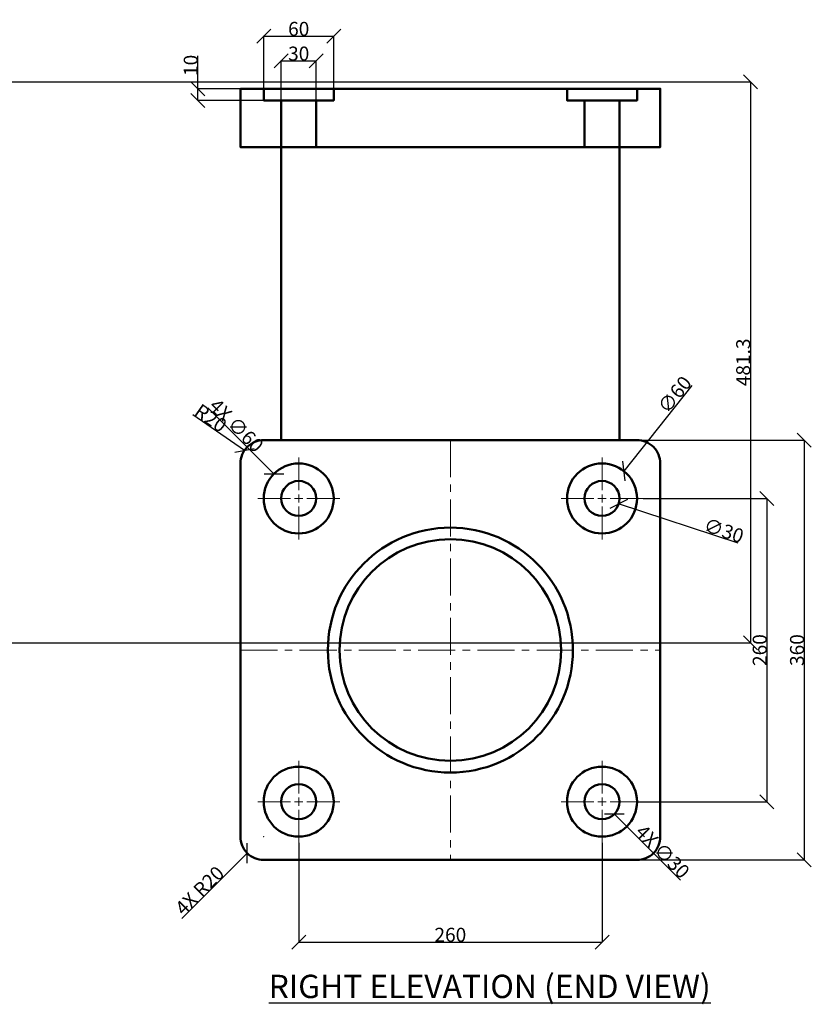
# Model space of a CAD drawing. Units: millimetres. Extents: x 509 to 2033, y 349 to 1731.
# Tile 2 of 2: x 1355 to 2033, y 349 to 1193. Entities that reach past the tile are written whole.
import ezdxf

# ---------------------------------------------------------------- set-up
doc = ezdxf.new("R2010")
doc.units = ezdxf.units.MM
doc.header["$MEASUREMENT"] = 0
doc.linetypes.add('CENTER', pattern=[50.8, 31.75, -6.35, 6.35, -6.35])
for name, color, linetype, lineweight in [('M-CNTR', 1, 'CENTER', 18), ('M-DIMS', 2, 'Continuous', 25), ('M-OUTL', 7, 'Continuous', 50), ('M-TEXT', 7, 'Continuous', 25)]:
    doc.layers.add(name, color=color, linetype=linetype, lineweight=lineweight)
doc.styles.get("Standard").update_dxf_attribs({"font": 'arial.ttf'})
doc.dimstyles.get("Standard").update_dxf_attribs({"dimtxt": 12, "dimasz": 12, "dimexe": 0.18, "dimexo": 0.0625, "dimgap": 0.09, "dimtad": 1, "dimdec": 0, "dimzin": 0, "dimdsep": 46, "dimtxsty": 'Standard', "dimblk": 'OBLIQUE', "dimcen": 0.09, "dimclre": 251, "dimadec": 0, "dimazin": 0, "dimtfac": 1, "dimtdec": 0, "dimtofl": 0, "dimtmove": 0, "dimatfit": 3, "dimfxl": 1, "dimtolj": 1, "dimtzin": 0, "dimarcsym": 0})

# ---------------------------------------------------------------- blocks, each defined once
blk = doc.blocks.new('*U6')
at = {"layer": 'M-CNTR', "color": 0, "transparency": 16777216}
for p, q in [((0, 7), (0, 35.12)), ((-35.12, 0), (-7, 0)), ((7, 0), (35.12, 0)), ((0, -35.12), (0, -7))]:
    blk.add_line(p, q, dxfattribs=at)
at = {"layer": 'M-CNTR', "color": 0, "linetype": 'Continuous', "transparency": 16777216}
for p, q in [((-3.5, 0), (3.5, 0)), ((0, -3.5), (0, 3.5))]:
    blk.add_line(p, q, dxfattribs=at)
blk = doc.blocks.new('*U7')
at = {"layer": 'M-CNTR', "color": 0, "transparency": 16777216}
for p, q in [((0, 7), (0, 35.12)), ((-35.12, 0), (-7, 0)), ((7, 0), (35.12, 0)), ((0, -35.12), (0, -7))]:
    blk.add_line(p, q, dxfattribs=at)
at = {"layer": 'M-CNTR', "color": 0, "linetype": 'Continuous', "transparency": 16777216}
for p, q in [((-3.5, 0), (3.5, 0)), ((0, -3.5), (0, 3.5))]:
    blk.add_line(p, q, dxfattribs=at)
blk = doc.blocks.new('*U8')
at = {"layer": 'M-CNTR', "color": 0, "transparency": 16777216}
for p, q in [((0, 7), (0, 35.12)), ((-35.12, 0), (-7, 0)), ((7, 0), (35.12, 0)), ((0, -35.12), (0, -7))]:
    blk.add_line(p, q, dxfattribs=at)
at = {"layer": 'M-CNTR', "color": 0, "linetype": 'Continuous', "transparency": 16777216}
for p, q in [((-3.5, 0), (3.5, 0)), ((0, -3.5), (0, 3.5))]:
    blk.add_line(p, q, dxfattribs=at)
blk = doc.blocks.new('*U9')
at = {"layer": 'M-CNTR', "color": 0, "transparency": 16777216}
for p, q in [((0, 7), (0, 35.12)), ((-35.12, 0), (-7, 0)), ((7, 0), (35.12, 0)), ((0, -35.12), (0, -7))]:
    blk.add_line(p, q, dxfattribs=at)
at = {"layer": 'M-CNTR', "color": 0, "linetype": 'Continuous', "transparency": 16777216}
for p, q in [((-3.5, 0), (3.5, 0)), ((0, -3.5), (0, 3.5))]:
    blk.add_line(p, q, dxfattribs=at)
blk = doc.blocks.new('_Oblique')
at = {"color": 0, "linetype": 'ByBlock', "lineweight": -2}
blk.add_line((-0.5, -0.5), (0.5, 0.5), dxfattribs=at)
blk = doc.blocks.new('*D25')
at = {"layer": 'Defpoints', "color": 0, "transparency": 16777216}
for p in [(1507.36, 1133.76), (1563.7, 1133.76), (1563.7, 1123.76)]:
    blk.add_point(p, dxfattribs=at)
at = {"layer": 'M-DIMS', "color": 0, "lineweight": -2, "transparency": 16777216}
for p, q in [((1507.36, 1133.76), (1507.36, 1161.96)), ((1563.64, 1133.76), (1507.18, 1133.76)), ((1507.36, 1123.76), (1507.36, 1133.76)), ((1563.64, 1123.76), (1507.18, 1123.76))]:
    blk.add_line(p, q, dxfattribs=at)
at = {"layer": 'M-DIMS', "color": 0, "lineweight": -2, "transparency": 16777216, "xscale": 12, "yscale": 12, "zscale": 12}
for p, rotation in [((1507.36, 1133.76), 90), ((1507.36, 1123.76), 270)]:
    blk.add_blockref('_Oblique', p, dxfattribs=dict(at, rotation=rotation))
at = {"layer": 'M-DIMS', "color": 0, "transparency": 16777216, "insert": (1501.14, 1153.86), "char_height": 12, "attachment_point": 5, "rotation": 90}
blk.add_mtext('\\A1;10', dxfattribs=at)
blk = doc.blocks.new('*D26')
at = {"layer": 'Defpoints', "color": 0, "transparency": 16777216}
for p in [(1623.7, 1178.95), (1563.7, 1133.76), (1623.7, 1133.76)]:
    blk.add_point(p, dxfattribs=at)
at = {"layer": 'M-DIMS', "color": 0, "lineweight": -2, "transparency": 16777216}
for p, q in [((1563.7, 1133.82), (1563.7, 1179.13)), ((1563.7, 1178.95), (1623.7, 1178.95)), ((1623.7, 1133.82), (1623.7, 1179.13))]:
    blk.add_line(p, q, dxfattribs=at)
at = {"layer": 'M-DIMS', "color": 0, "lineweight": -2, "transparency": 16777216, "xscale": 12, "yscale": 12, "zscale": 12, "rotation": 180}
blk.add_blockref('_Oblique', (1563.7, 1178.95), dxfattribs=at)
at = {"layer": 'M-DIMS', "color": 0, "lineweight": -2, "transparency": 16777216, "xscale": 12, "yscale": 12, "zscale": 12}
blk.add_blockref('_Oblique', (1623.7, 1178.95), dxfattribs=at)
at = {"layer": 'M-DIMS', "color": 0, "transparency": 16777216, "insert": (1593.7, 1185.16), "char_height": 12, "attachment_point": 5}
blk.add_mtext('\\A1;60', dxfattribs=at)
blk = doc.blocks.new('*D27')
at = {"layer": 'Defpoints', "color": 0, "transparency": 16777216}
for p in [(1608.7, 1157.75), (1578.7, 1123.76), (1608.7, 1123.76)]:
    blk.add_point(p, dxfattribs=at)
at = {"layer": 'M-DIMS', "color": 0, "lineweight": -2, "transparency": 16777216}
for p, q in [((1578.7, 1123.82), (1578.7, 1157.93)), ((1578.7, 1157.75), (1608.7, 1157.75)), ((1608.7, 1123.82), (1608.7, 1157.93))]:
    blk.add_line(p, q, dxfattribs=at)
at = {"layer": 'M-DIMS', "color": 0, "lineweight": -2, "transparency": 16777216, "xscale": 12, "yscale": 12, "zscale": 12, "rotation": 180}
blk.add_blockref('_Oblique', (1578.7, 1157.75), dxfattribs=at)
at = {"layer": 'M-DIMS', "color": 0, "lineweight": -2, "transparency": 16777216, "xscale": 12, "yscale": 12, "zscale": 12}
blk.add_blockref('_Oblique', (1608.7, 1157.75), dxfattribs=at)
at = {"layer": 'M-DIMS', "color": 0, "transparency": 16777216, "insert": (1593.7, 1163.97), "char_height": 12, "attachment_point": 5}
blk.add_mtext('\\A1;30', dxfattribs=at)
blk = doc.blocks.new('*D28')
at = {"layer": 'Defpoints', "color": 0, "transparency": 16777216}
for p in [(1872.35, 806.01), (1835.05, 759.01)]:
    blk.add_point(p, dxfattribs=at)
at = {"layer": 'M-DIMS', "color": 0, "lineweight": -2, "transparency": 16777216}
for p, q in [((1930.58, 879.38), (1872.35, 806.01)), ((1853.61, 782.51), (1853.79, 782.51)), ((1853.7, 782.42), (1853.7, 782.6))]:
    blk.add_line(p, q, dxfattribs=at)
at = {"layer": 'M-DIMS', "color": 0, "lineweight": -2, "transparency": 16777216, "xscale": 12, "yscale": 12, "zscale": 12, "rotation": 231.5643367967079}
blk.add_blockref('_Oblique', (1872.35, 806.01), dxfattribs=at)
at = {"layer": 'M-DIMS', "color": 0, "transparency": 16777216, "insert": (1916.01, 871.56), "char_height": 12, "attachment_point": 5, "rotation": 51.56434}
blk.add_mtext('\\A1;∅60', dxfattribs=at)
blk = doc.blocks.new('*D29')
at = {"layer": 'Defpoints', "color": 0, "transparency": 16777216}
for p in [(1839.45, 787.2), (1867.95, 777.81)]:
    blk.add_point(p, dxfattribs=at)
at = {"layer": 'M-DIMS', "color": 0, "lineweight": -2, "transparency": 16777216}
for p, q in [((1853.61, 782.51), (1853.79, 782.51)), ((1853.7, 782.42), (1853.7, 782.6)), ((1970.52, 744.04), (1867.95, 777.81))]:
    blk.add_line(p, q, dxfattribs=at)
at = {"layer": 'M-DIMS', "color": 0, "lineweight": -2, "transparency": 16777216, "xscale": 12, "yscale": 12, "zscale": 12, "rotation": 161.7757335580119}
blk.add_blockref('_Oblique', (1867.95, 777.81), dxfattribs=at)
at = {"layer": 'M-DIMS', "color": 0, "transparency": 16777216, "insert": (1958.14, 755.02), "char_height": 12, "attachment_point": 5, "rotation": 341.77573}
blk.add_mtext('\\A1;∅30', dxfattribs=at)
blk = doc.blocks.new('*D30')
at = {"layer": 'Defpoints', "color": 0, "transparency": 16777216}
for p in [(1547.24, 823.87), (1563.7, 812.51)]:
    blk.add_point(p, dxfattribs=at)
at = {"layer": 'M-DIMS', "color": 0, "lineweight": -2, "transparency": 16777216}
for p, q in [((1502.91, 854.49), (1547.24, 823.87)), ((1563.61, 812.51), (1563.79, 812.51)), ((1563.7, 812.42), (1563.7, 812.6))]:
    blk.add_line(p, q, dxfattribs=at)
at = {"layer": 'M-DIMS', "color": 0, "lineweight": -2, "transparency": 16777216, "xscale": 12, "yscale": 12, "zscale": 12, "rotation": 325.3742134836517}
blk.add_blockref('_Oblique', (1547.24, 823.87), dxfattribs=at)
at = {"layer": 'M-DIMS', "color": 0, "transparency": 16777216, "insert": (1518.29, 851.42), "char_height": 12, "attachment_point": 5, "rotation": 325.37421}
blk.add_mtext('\\A1;R20', dxfattribs=at)
blk = doc.blocks.new('*D31')
at = {"layer": 'Defpoints', "color": 0, "transparency": 16777216}
for p in [(1593.7, 487.39), (1853.7, 487.39), (1853.7, 402.15)]:
    blk.add_point(p, dxfattribs=at)
at = {"layer": 'M-DIMS', "color": 0, "lineweight": -2, "transparency": 16777216}
for p, q in [((1593.7, 487.32), (1593.7, 401.97)), ((1853.7, 487.32), (1853.7, 401.97)), ((1593.7, 402.15), (1853.7, 402.15))]:
    blk.add_line(p, q, dxfattribs=at)
at = {"layer": 'M-DIMS', "color": 0, "lineweight": -2, "transparency": 16777216, "xscale": 12, "yscale": 12, "zscale": 12, "rotation": 180}
blk.add_blockref('_Oblique', (1593.7, 402.15), dxfattribs=at)
at = {"layer": 'M-DIMS', "color": 0, "lineweight": -2, "transparency": 16777216, "xscale": 12, "yscale": 12, "zscale": 12}
blk.add_blockref('_Oblique', (1853.7, 402.15), dxfattribs=at)
at = {"layer": 'M-DIMS', "color": 0, "transparency": 16777216, "insert": (1723.7, 408.37), "char_height": 12, "attachment_point": 5}
blk.add_mtext('\\A1;260', dxfattribs=at)
blk = doc.blocks.new('*D32')
at = {"layer": 'Defpoints', "color": 0, "transparency": 16777216}
for p in [(1888.82, 782.51), (1883.7, 522.51), (1995.11, 522.51)]:
    blk.add_point(p, dxfattribs=at)
at = {"layer": 'M-DIMS', "color": 0, "lineweight": -2, "transparency": 16777216}
for p, q in [((1888.88, 782.51), (1995.29, 782.51)), ((1995.11, 782.51), (1995.11, 522.51)), ((1883.76, 522.51), (1995.29, 522.51))]:
    blk.add_line(p, q, dxfattribs=at)
at = {"layer": 'M-DIMS', "color": 0, "lineweight": -2, "transparency": 16777216, "xscale": 12, "yscale": 12, "zscale": 12}
for p, rotation in [((1995.11, 782.51), 90), ((1995.11, 522.51), 270)]:
    blk.add_blockref('_Oblique', p, dxfattribs=dict(at, rotation=rotation))
at = {"layer": 'M-DIMS', "color": 0, "transparency": 16777216, "insert": (1988.9, 652.51), "char_height": 12, "attachment_point": 5, "rotation": 90}
blk.add_mtext('\\A1;260', dxfattribs=at)
blk = doc.blocks.new('*D33')
at = {"layer": 'Defpoints', "color": 0, "transparency": 16777216}
for p in [(1883.7, 832.51), (1883.7, 472.51), (2027.12, 472.51)]:
    blk.add_point(p, dxfattribs=at)
at = {"layer": 'M-DIMS', "color": 0, "lineweight": -2, "transparency": 16777216}
for p, q in [((1883.76, 832.51), (2027.3, 832.51)), ((2027.12, 832.51), (2027.12, 472.51)), ((1883.76, 472.51), (2027.3, 472.51))]:
    blk.add_line(p, q, dxfattribs=at)
at = {"layer": 'M-DIMS', "color": 0, "lineweight": -2, "transparency": 16777216, "xscale": 12, "yscale": 12, "zscale": 12}
for p, rotation in [((2027.12, 832.51), 90), ((2027.12, 472.51), 270)]:
    blk.add_blockref('_Oblique', p, dxfattribs=dict(at, rotation=rotation))
at = {"layer": 'M-DIMS', "color": 0, "transparency": 16777216, "insert": (2020.9, 652.51), "char_height": 12, "attachment_point": 5, "rotation": 90}
blk.add_mtext('\\A1;360', dxfattribs=at)
blk = doc.blocks.new('BOLT-HOLE-CBORE')
for radius in [30, 15]:
    blk.add_circle((30, 30), radius)
blk = doc.blocks.new('*D35')
at = {"layer": 'Defpoints', "color": 0, "transparency": 16777216}
for p in [(968.18, 1139.86), (1240.92, 658.61), (1980.95, 658.61)]:
    blk.add_point(p, dxfattribs=at)
at = {"layer": 'M-DIMS', "color": 251, "lineweight": -2, "transparency": 16777216}
for p, q in [((968.24, 1139.86), (1981.13, 1139.86)), ((1240.98, 658.61), (1981.13, 658.61))]:
    blk.add_line(p, q, dxfattribs=at)
at = {"layer": 'M-DIMS', "color": 0, "lineweight": -2, "transparency": 16777216}
blk.add_line((1980.95, 1139.86), (1980.95, 658.61), dxfattribs=at)
at = {"layer": 'M-DIMS', "color": 0, "lineweight": -2, "transparency": 16777216, "xscale": 12, "yscale": 12, "zscale": 12}
for p, rotation in [((1980.95, 1139.86), 90), ((1980.95, 658.61), 270)]:
    blk.add_blockref('_Oblique', p, dxfattribs=dict(at, rotation=rotation))
at = {"layer": 'M-DIMS', "color": 0, "transparency": 16777216, "insert": (1974.73, 899.23), "char_height": 12, "attachment_point": 5, "rotation": 90}
blk.add_mtext('\\A1;481.3', dxfattribs=at)
blk = doc.blocks.new('*D42')
at = {"layer": 'Defpoints', "color": 0, "transparency": 16777216}
for p in [(1572.48, 803.72), (1614.92, 761.3)]:
    blk.add_point(p, dxfattribs=at)
at = {"layer": 'M-DIMS', "color": 0, "lineweight": -2, "transparency": 16777216}
blk.add_line((1515.9, 860.28), (1572.48, 803.72), dxfattribs=at)
at = {"layer": 'M-DIMS', "color": 251, "lineweight": -2, "transparency": 16777216}
for p, q in [((1593.61, 782.51), (1593.79, 782.51)), ((1593.7, 782.42), (1593.7, 782.6))]:
    blk.add_line(p, q, dxfattribs=at)
at = {"layer": 'M-DIMS', "color": 0, "lineweight": -2, "transparency": 16777216, "xscale": 12, "yscale": 12, "zscale": 12, "rotation": 315.010169072893}
blk.add_blockref('_Oblique', (1572.48, 803.72), dxfattribs=at)
at = {"layer": 'M-DIMS', "color": 0, "transparency": 16777216, "insert": (1540.34, 845.12), "char_height": 12, "attachment_point": 5, "rotation": 315.01017}
blk.add_mtext('\\A1;4X ∅60', dxfattribs=at)
blk = doc.blocks.new('*D43')
at = {"layer": 'Defpoints', "color": 0, "transparency": 16777216}
for p in [(1843.1, 533.12), (1864.3, 511.9)]:
    blk.add_point(p, dxfattribs=at)
at = {"layer": 'M-DIMS', "color": 251, "lineweight": -2, "transparency": 16777216}
for p, q in [((1853.61, 522.51), (1853.79, 522.51)), ((1853.7, 522.42), (1853.7, 522.6))]:
    blk.add_line(p, q, dxfattribs=at)
at = {"layer": 'M-DIMS', "color": 0, "lineweight": -2, "transparency": 16777216}
blk.add_line((1920.86, 455.3), (1864.3, 511.9), dxfattribs=at)
at = {"layer": 'M-DIMS', "color": 0, "lineweight": -2, "transparency": 16777216, "xscale": 12, "yscale": 12, "zscale": 12, "rotation": 134.9796672557942}
blk.add_blockref('_Oblique', (1864.3, 511.9), dxfattribs=at)
at = {"layer": 'M-DIMS', "color": 0, "transparency": 16777216, "insert": (1905.7, 479.74), "char_height": 12, "attachment_point": 5, "rotation": 314.97967}
blk.add_mtext('\\A1;4X ∅30', dxfattribs=at)
blk = doc.blocks.new('*D44')
at = {"layer": 'Defpoints', "color": 0, "transparency": 16777216}
for p in [(1563.7, 492.51), (1549.56, 478.36)]:
    blk.add_point(p, dxfattribs=at)
at = {"layer": 'M-DIMS', "color": 251, "lineweight": -2, "transparency": 16777216}
for p, q in [((1563.61, 492.51), (1563.79, 492.51)), ((1563.7, 492.42), (1563.7, 492.6))]:
    blk.add_line(p, q, dxfattribs=at)
at = {"layer": 'M-DIMS', "color": 0, "lineweight": -2, "transparency": 16777216}
blk.add_line((1493.65, 422.44), (1549.56, 478.36), dxfattribs=at)
at = {"layer": 'M-DIMS', "color": 0, "lineweight": -2, "transparency": 16777216, "xscale": 12, "yscale": 12, "zscale": 12, "rotation": 45.00836011224599}
blk.add_blockref('_Oblique', (1549.56, 478.36), dxfattribs=at)
at = {"layer": 'M-DIMS', "color": 0, "transparency": 16777216, "insert": (1508.73, 446.31), "char_height": 12, "attachment_point": 5, "rotation": 45.00836}
blk.add_mtext('\\A1;4X R20', dxfattribs=at)

msp = doc.modelspace()

# ---------------------------------------------------------------- linework, layer by layer
at = {"layer": 'M-CNTR'}
for p, q in [((1723.7, 832.51), (1723.7, 472.51)), ((1543.7, 652.51), (1903.7, 652.51))]:
    msp.add_line(p, q, dxfattribs=at)
at = {"layer": 'M-OUTL'}
for p, q in [((1578.7, 1123.76), (1578.7, 832.51)), ((1608.7, 1123.76), (1608.7, 1083.76)), ((1838.7, 1083.76), (1838.7, 1123.76)), ((1868.7, 1123.76), (1868.7, 832.51))]:
    msp.add_line(p, q, dxfattribs=at)
for points in [[(1543.7, 1133.76), (1903.7, 1133.76), (1903.7, 1083.76), (1543.7, 1083.76)], [(1563.7, 1133.76), (1623.7, 1133.76), (1623.7, 1123.76), (1563.7, 1123.76)], [(1823.7, 1133.76), (1883.7, 1133.76), (1883.7, 1123.76), (1823.7, 1123.76)]]:
    msp.add_lwpolyline(points, close=True, dxfattribs=at)
msp.add_lwpolyline([(1563.7, 832.51), (1883.7, 832.51, -0.414214), (1903.7, 812.51), (1903.7, 492.51, -0.414214), (1883.7, 472.51), (1563.7, 472.51, -0.414214), (1543.7, 492.51), (1543.7, 812.51, -0.414214)], format="xyb", close=True, dxfattribs=at)
for centre, radius in [((1593.7, 782.51), 30), ((1723.7, 652.51), 105), ((1723.7, 652.51), 95)]:
    msp.add_circle(centre, radius, dxfattribs=at)

# ---------------------------------------------------------------- block references
at = {"layer": 'M-CNTR'}
for name, p in [('*U8', (1593.7, 782.51)), ('*U9', (1853.7, 782.51)), ('*U7', (1593.7, 522.51)), ('*U6', (1853.7, 522.51))]:
    msp.add_blockref(name, p, dxfattribs=at)
at = {"layer": 'M-OUTL'}
for p in [(1563.7, 752.51), (1823.7, 752.51), (1563.7, 492.51), (1823.7, 492.51)]:
    msp.add_blockref('BOLT-HOLE-CBORE', p, dxfattribs=at)

# ---------------------------------------------------------------- texts
at = {"layer": 'M-TEXT', "insert": (1757.42, 364.11), "char_height": 20, "attachment_point": 5}
msp.add_mtext('\\A1;{\\LRIGHT ELEVATION (END VIEW)}', dxfattribs=at)

# ---------------------------------------------------------------- dimensions: what is measured, and where the dimension line sits
at = {"layer": 'M-DIMS'}
for base, p1, p2, picture, middle in [((1623.7, 1178.95), (1563.7, 1133.76), (1623.7, 1133.76), '*D26', (1593.7, 1185.16)), ((1608.7, 1157.75), (1578.7, 1123.76), (1608.7, 1123.76), '*D27', (1593.7, 1163.97)), ((1853.7, 402.15), (1593.7, 487.39), (1853.7, 487.39), '*D31', (1723.7, 408.37))]:
    dim = msp.add_linear_dim(base=base, p1=p1, p2=p2, dimstyle='Standard', override={"dimclrd": 0, "dimclre": 0, "dimclrt": 0}, dxfattribs=at)
    dim.commit()
    dim.dimension.update_dxf_attribs({"geometry": picture, "text_midpoint": middle})
for base, p1, p2, override, picture, middle in [((1507.36, 1133.76), (1563.7, 1123.76), (1563.7, 1133.76), {"dimclrd": 0, "dimclre": 0, "dimclrt": 0}, '*D25', (1501.14, 1153.86)), ((1980.9517, 658.6051), (968.1801, 1139.8615), (1240.9212, 658.6051), {"dimdec": 1, "dimlfac": 1, "dimrnd": 0, "dimzin": 0, "dimdsep": 46, "dimlunit": 2}, '*D35', (1974.7307, 899.2333)), ((2027.12, 472.51), (1883.7, 832.51), (1883.7, 472.51), {"dimclrd": 0, "dimclre": 0, "dimclrt": 0}, '*D33', (2020.9, 652.51)), ((1995.11, 522.51), (1888.82, 782.51), (1883.7, 522.51), {"dimclrd": 0, "dimclre": 0, "dimclrt": 0}, '*D32', (1988.9, 652.51))]:
    dim = msp.add_linear_dim(base=base, p1=p1, p2=p2, angle=90, dimstyle='Standard', override=override, dxfattribs=at)
    dim.commit()
    dim.dimension.update_dxf_attribs({"geometry": picture, "text_midpoint": middle})
for p1, p2, picture, middle in [((1835.05, 759.01), (1872.35, 806.01), '*D28', (1921.14, 867.48)), ((1839.45, 787.2), (1867.95, 777.81), '*D29', (1956.09, 748.79))]:
    dim = msp.add_diameter_dim_2p(p1=p1, p2=p2, dimstyle='Standard', override={"dimclrd": 0, "dimclre": 0, "dimclrt": 0}, dxfattribs=at)
    dim.commit()
    dim.dimension.update_dxf_attribs({"geometry": picture, "text_midpoint": middle, "dimtype": 163})
for p1, p2, picture, middle in [((1614.92, 761.3), (1572.48, 803.72), '*D42', (1535.7, 840.48)), ((1843.1, 533.12), (1864.3, 511.9), '*D43', (1901.07, 475.11))]:
    dim = msp.add_diameter_dim_2p(p1=p1, p2=p2, text='4X <>', dimstyle='Standard', override={"dimdec": 0, "dimlfac": 1, "dimrnd": 0, "dimzin": 0, "dimdsep": 46, "dimlunit": 2}, dxfattribs=at)
    dim.commit()
    dim.dimension.update_dxf_attribs({"geometry": picture, "text_midpoint": middle, "dimtype": 163})
dim = msp.add_radius_dim(center=(1563.7, 812.51), mpoint=(1547.24, 823.87), dimstyle='Standard', override={"dimclrd": 0, "dimclre": 0, "dimclrt": 0}, dxfattribs=at)
dim.commit()
dim.dimension.update_dxf_attribs({"geometry": '*D30', "text_midpoint": (1514.76, 846.3), "dimtype": 164})
dim = msp.add_radius_dim(center=(1563.7, 492.51), mpoint=(1549.56, 478.36), text='4X <>', dimstyle='Standard', override={"dimdec": 0, "dimlfac": 1, "dimrnd": 0, "dimzin": 0, "dimdsep": 46, "dimlunit": 2}, dxfattribs=at)
dim.commit()
dim.dimension.update_dxf_attribs({"geometry": '*D44', "text_midpoint": (1508.73, 446.31)})

doc.saveas('drawing.dxf')
